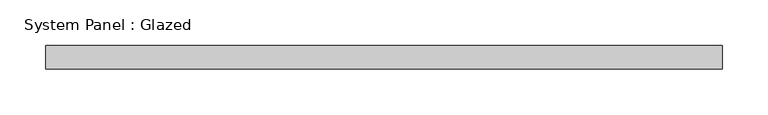
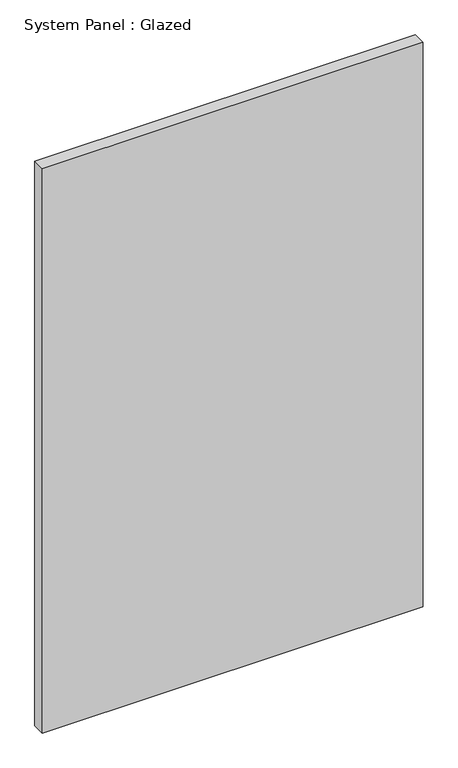
"""IFC4 building model written with IfcOpenShell, lengths in millimetres: plate geometry, System Panel : Glazed."""

from ifc_helpers import new_model, si_unit, origin, origin_with_axes, place, context, project, spatial, polyline, outline, extrude, source, transform, mapped, element, save


def system_panel_glazed_904ef9a5(model_context):
    return source(origin(), model_context, "Body", "SweptSolid", [
        extrude(outline(polyline([(368.6978183, 19.05), (-368.6978183, 19.05), (-368.6978183, 44.45), (368.6978183, 44.45), (368.6978183, 19.05)])), origin_with_axes(), (0.0, 0.0, 1.0), 1155.7),
    ])


if __name__ == "__main__":
    model = new_model("IFC4")
    model_context = context("Model", 3, world=origin())
    ifc_project = project(units=[si_unit("LENGTHUNIT", "METRE", prefix="MILLI")], contexts=[model_context])
    site = spatial("IfcSite", under=ifc_project)
    building = spatial("IfcBuilding", under=site)
    placement = place(None, origin())
    system_panel_glazed_shape = system_panel_glazed_904ef9a5(model_context)
    element("IfcPlate", 1, ObjectType="System Panel : Glazed", at=placement, inside=building, context=model_context, shape_type="MappedRepresentation", body=[
        mapped(system_panel_glazed_shape, transform((0.0, 0.0, 0.0), x_axis=(1.0, 0.0, 0.0), y_axis=(0.0, 1.0, 0.0), z_axis=(0.0, 0.0, 1.0))),
    ])
    save(model, "model.ifc")

# Revit data of these elements
# Type "System Panel : Glazed"
#   Construction Type Id = "GSP4R"
#   Analytic Construction = "1/8 in Pilkington single glazing"
#   Visual Light Transmittance = 0.9
#   Solar Heat Gain Coefficient = 0.86
#   Heat Transfer Coefficient (U) = 1.18115 BTU/(h·ft²·°F)
# Element 1 (IfcPlate, "System Panel : Glazed")
#   Materials on its faces: "Glass"
# Materials
#   "Glass": class "Glass", colour RGB 0 128 192, transparency 0.75, Description = "Soda Lime Glass", Cost = 0
